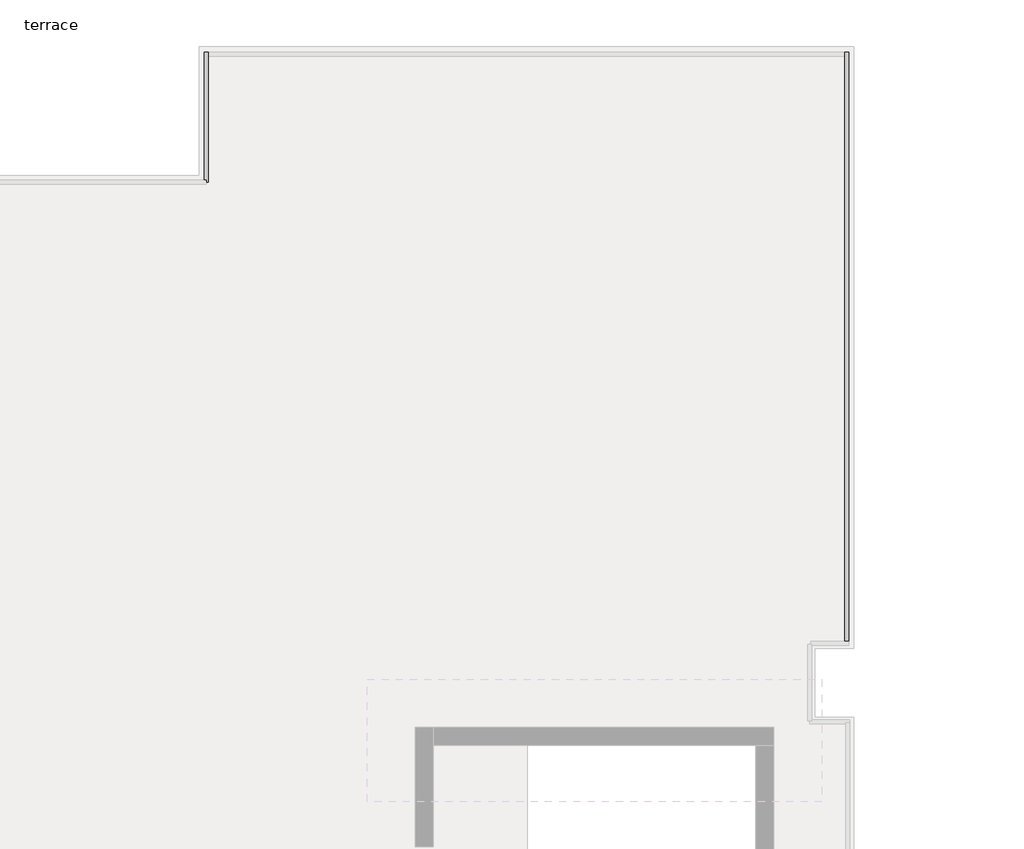
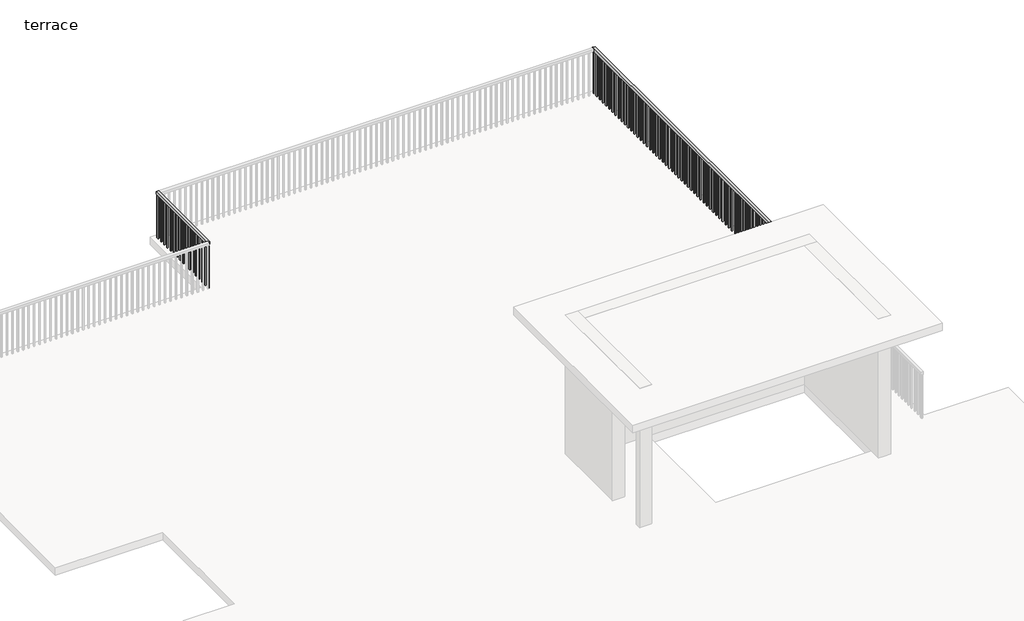
# One storey, part 6 of 7: 2 railings.
"""IFC4 building model written with IfcOpenShell, lengths in millimetres."""

from ifc_helpers import new_model, si_unit, frame, origin, place, context, project, spatial, polyline, outline, extrude, element, save

model = new_model("IFC4")

# Units and contexts
model_context = context("Model", 3, world=origin())
ifc_project = project(units=[si_unit("LENGTHUNIT", "METRE", prefix="MILLI")], contexts=[model_context])

# Site, building, storey
site = spatial("IfcSite", under=ifc_project)
building = spatial("IfcBuilding", under=site)
storey = spatial("IfcBuildingStorey", under=building, Name="terrace", Elevation=3810.0)

# Railings
placement = place(None, origin())
element("IfcRailing", 1, ObjectType="Handrail - Rectangular", at=placement, inside=storey, context=model_context, shape_type="SweptSolid", body=[
    extrude(outline(polyline([(-8384.4890129, 11008.027622), (-8435.2890129, 11008.027622), (-8435.2890129, 12659.027622), (-8384.4890129, 12659.027622), (-8384.4890129, 11008.027622)])), frame((0.0, 0.0, 4673.6), z_axis=(0.0, 0.0, 1.0), x_axis=(1.0, 0.0, 0.0)), (0.0, 0.0, 1.0), 50.8),
    extrude(outline(polyline([(-8400.3640129, 12624.102622), (-8419.4140129, 12624.102622), (-8419.4140129, 12643.152622), (-8400.3640129, 12643.152622), (-8400.3640129, 12624.102622)])), frame((0.0, 0.0, 3810.0), z_axis=(0.0, 0.0, 1.0), x_axis=(1.0, 0.0, 0.0)), (0.0, 0.0, 1.0), 863.6),
    extrude(outline(polyline([(-8400.3640129, 12522.502622), (-8419.4140129, 12522.502622), (-8419.4140129, 12541.552622), (-8400.3640129, 12541.552622), (-8400.3640129, 12522.502622)])), frame((0.0, 0.0, 3810.0), z_axis=(0.0, 0.0, 1.0), x_axis=(1.0, 0.0, 0.0)), (0.0, 0.0, 1.0), 863.6),
    extrude(outline(polyline([(-8400.3640129, 12420.902622), (-8419.4140129, 12420.902622), (-8419.4140129, 12439.952622), (-8400.3640129, 12439.952622), (-8400.3640129, 12420.902622)])), frame((0.0, 0.0, 3810.0), z_axis=(0.0, 0.0, 1.0), x_axis=(1.0, 0.0, 0.0)), (0.0, 0.0, 1.0), 863.6),
    extrude(outline(polyline([(-8400.3640129, 12319.302622), (-8419.4140129, 12319.302622), (-8419.4140129, 12338.352622), (-8400.3640129, 12338.352622), (-8400.3640129, 12319.302622)])), frame((0.0, 0.0, 3810.0), z_axis=(0.0, 0.0, 1.0), x_axis=(1.0, 0.0, 0.0)), (0.0, 0.0, 1.0), 863.6),
    extrude(outline(polyline([(-8400.3640129, 12217.702622), (-8419.4140129, 12217.702622), (-8419.4140129, 12236.752622), (-8400.3640129, 12236.752622), (-8400.3640129, 12217.702622)])), frame((0.0, 0.0, 3810.0), z_axis=(0.0, 0.0, 1.0), x_axis=(1.0, 0.0, 0.0)), (0.0, 0.0, 1.0), 863.6),
    extrude(outline(polyline([(-8400.3640129, 12116.102622), (-8419.4140129, 12116.102622), (-8419.4140129, 12135.152622), (-8400.3640129, 12135.152622), (-8400.3640129, 12116.102622)])), frame((0.0, 0.0, 3810.0), z_axis=(0.0, 0.0, 1.0), x_axis=(1.0, 0.0, 0.0)), (0.0, 0.0, 1.0), 863.6),
    extrude(outline(polyline([(-8400.3640129, 12014.502622), (-8419.4140129, 12014.502622), (-8419.4140129, 12033.552622), (-8400.3640129, 12033.552622), (-8400.3640129, 12014.502622)])), frame((0.0, 0.0, 3810.0), z_axis=(0.0, 0.0, 1.0), x_axis=(1.0, 0.0, 0.0)), (0.0, 0.0, 1.0), 863.6),
    extrude(outline(polyline([(-8400.3640129, 11912.902622), (-8419.4140129, 11912.902622), (-8419.4140129, 11931.952622), (-8400.3640129, 11931.952622), (-8400.3640129, 11912.902622)])), frame((0.0, 0.0, 3810.0), z_axis=(0.0, 0.0, 1.0), x_axis=(1.0, 0.0, 0.0)), (0.0, 0.0, 1.0), 863.6),
    extrude(outline(polyline([(-8400.3640129, 11811.302622), (-8419.4140129, 11811.302622), (-8419.4140129, 11830.352622), (-8400.3640129, 11830.352622), (-8400.3640129, 11811.302622)])), frame((0.0, 0.0, 3810.0), z_axis=(0.0, 0.0, 1.0), x_axis=(1.0, 0.0, 0.0)), (0.0, 0.0, 1.0), 863.6),
    extrude(outline(polyline([(-8400.3640129, 11709.702622), (-8419.4140129, 11709.702622), (-8419.4140129, 11728.752622), (-8400.3640129, 11728.752622), (-8400.3640129, 11709.702622)])), frame((0.0, 0.0, 3810.0), z_axis=(0.0, 0.0, 1.0), x_axis=(1.0, 0.0, 0.0)), (0.0, 0.0, 1.0), 863.6),
    extrude(outline(polyline([(-8400.3640129, 11608.102622), (-8419.4140129, 11608.102622), (-8419.4140129, 11627.152622), (-8400.3640129, 11627.152622), (-8400.3640129, 11608.102622)])), frame((0.0, 0.0, 3810.0), z_axis=(0.0, 0.0, 1.0), x_axis=(1.0, 0.0, 0.0)), (0.0, 0.0, 1.0), 863.6),
    extrude(outline(polyline([(-8400.3640129, 11506.502622), (-8419.4140129, 11506.502622), (-8419.4140129, 11525.552622), (-8400.3640129, 11525.552622), (-8400.3640129, 11506.502622)])), frame((0.0, 0.0, 3810.0), z_axis=(0.0, 0.0, 1.0), x_axis=(1.0, 0.0, 0.0)), (0.0, 0.0, 1.0), 863.6),
    extrude(outline(polyline([(-8400.3640129, 11404.902622), (-8419.4140129, 11404.902622), (-8419.4140129, 11423.952622), (-8400.3640129, 11423.952622), (-8400.3640129, 11404.902622)])), frame((0.0, 0.0, 3810.0), z_axis=(0.0, 0.0, 1.0), x_axis=(1.0, 0.0, 0.0)), (0.0, 0.0, 1.0), 863.6),
    extrude(outline(polyline([(-8400.3640129, 11303.302622), (-8419.4140129, 11303.302622), (-8419.4140129, 11322.352622), (-8400.3640129, 11322.352622), (-8400.3640129, 11303.302622)])), frame((0.0, 0.0, 3810.0), z_axis=(0.0, 0.0, 1.0), x_axis=(1.0, 0.0, 0.0)), (0.0, 0.0, 1.0), 863.6),
    extrude(outline(polyline([(-8400.3640129, 11201.702622), (-8419.4140129, 11201.702622), (-8419.4140129, 11220.752622), (-8400.3640129, 11220.752622), (-8400.3640129, 11201.702622)])), frame((0.0, 0.0, 3810.0), z_axis=(0.0, 0.0, 1.0), x_axis=(1.0, 0.0, 0.0)), (0.0, 0.0, 1.0), 863.6),
    extrude(outline(polyline([(-8400.3640129, 11100.102622), (-8419.4140129, 11100.102622), (-8419.4140129, 11119.152622), (-8400.3640129, 11119.152622), (-8400.3640129, 11100.102622)])), frame((0.0, 0.0, 3810.0), z_axis=(0.0, 0.0, 1.0), x_axis=(1.0, 0.0, 0.0)), (0.0, 0.0, 1.0), 863.6),
    extrude(outline(polyline([(-8400.3640129, 12639.977622), (-8419.4140129, 12639.977622), (-8419.4140129, 12659.027622), (-8400.3640129, 12659.027622), (-8400.3640129, 12639.977622)])), frame((0.0, 0.0, 3810.0), z_axis=(0.0, 0.0, 1.0), x_axis=(1.0, 0.0, 0.0)), (0.0, 0.0, 1.0), 863.6),
    extrude(outline(polyline([(-8400.3640129, 11008.027622), (-8419.4140129, 11008.027622), (-8419.4140129, 11027.077622), (-8400.3640129, 11027.077622), (-8400.3640129, 11008.027622)])), frame((0.0, 0.0, 3810.0), z_axis=(0.0, 0.0, 1.0), x_axis=(1.0, 0.0, 0.0)), (0.0, 0.0, 1.0), 863.6),
])
element("IfcRailing", 2, ObjectType="Handrail - Rectangular", at=placement, inside=storey, context=model_context, shape_type="SweptSolid", body=[
    extrude(outline(polyline([(-307.2890129, 12659.027622), (-256.4890129, 12659.027622), (-256.4890129, 5140.627622), (-307.2890129, 5140.627622), (-307.2890129, 12659.027622)])), frame((0.0, 0.0, 4673.6), z_axis=(0.0, 0.0, 1.0), x_axis=(1.0, 0.0, 0.0)), (0.0, 0.0, 1.0), 50.8),
    extrude(outline(polyline([(-291.4140129, 5251.752622), (-272.3640129, 5251.752622), (-272.3640129, 5232.702622), (-291.4140129, 5232.702622), (-291.4140129, 5251.752622)])), frame((0.0, 0.0, 3810.0), z_axis=(0.0, 0.0, 1.0), x_axis=(1.0, 0.0, 0.0)), (0.0, 0.0, 1.0), 863.6),
    extrude(outline(polyline([(-291.4140129, 5353.352622), (-272.3640129, 5353.352622), (-272.3640129, 5334.302622), (-291.4140129, 5334.302622), (-291.4140129, 5353.352622)])), frame((0.0, 0.0, 3810.0), z_axis=(0.0, 0.0, 1.0), x_axis=(1.0, 0.0, 0.0)), (0.0, 0.0, 1.0), 863.6),
    extrude(outline(polyline([(-291.4140129, 5454.952622), (-272.3640129, 5454.952622), (-272.3640129, 5435.902622), (-291.4140129, 5435.902622), (-291.4140129, 5454.952622)])), frame((0.0, 0.0, 3810.0), z_axis=(0.0, 0.0, 1.0), x_axis=(1.0, 0.0, 0.0)), (0.0, 0.0, 1.0), 863.6),
    extrude(outline(polyline([(-291.4140129, 5556.552622), (-272.3640129, 5556.552622), (-272.3640129, 5537.502622), (-291.4140129, 5537.502622), (-291.4140129, 5556.552622)])), frame((0.0, 0.0, 3810.0), z_axis=(0.0, 0.0, 1.0), x_axis=(1.0, 0.0, 0.0)), (0.0, 0.0, 1.0), 863.6),
    extrude(outline(polyline([(-291.4140129, 5658.152622), (-272.3640129, 5658.152622), (-272.3640129, 5639.102622), (-291.4140129, 5639.102622), (-291.4140129, 5658.152622)])), frame((0.0, 0.0, 3810.0), z_axis=(0.0, 0.0, 1.0), x_axis=(1.0, 0.0, 0.0)), (0.0, 0.0, 1.0), 863.6),
    extrude(outline(polyline([(-291.4140129, 5759.752622), (-272.3640129, 5759.752622), (-272.3640129, 5740.702622), (-291.4140129, 5740.702622), (-291.4140129, 5759.752622)])), frame((0.0, 0.0, 3810.0), z_axis=(0.0, 0.0, 1.0), x_axis=(1.0, 0.0, 0.0)), (0.0, 0.0, 1.0), 863.6),
    extrude(outline(polyline([(-291.4140129, 5861.352622), (-272.3640129, 5861.352622), (-272.3640129, 5842.302622), (-291.4140129, 5842.302622), (-291.4140129, 5861.352622)])), frame((0.0, 0.0, 3810.0), z_axis=(0.0, 0.0, 1.0), x_axis=(1.0, 0.0, 0.0)), (0.0, 0.0, 1.0), 863.6),
    extrude(outline(polyline([(-291.4140129, 5962.952622), (-272.3640129, 5962.952622), (-272.3640129, 5943.902622), (-291.4140129, 5943.902622), (-291.4140129, 5962.952622)])), frame((0.0, 0.0, 3810.0), z_axis=(0.0, 0.0, 1.0), x_axis=(1.0, 0.0, 0.0)), (0.0, 0.0, 1.0), 863.6),
    extrude(outline(polyline([(-291.4140129, 6064.552622), (-272.3640129, 6064.552622), (-272.3640129, 6045.502622), (-291.4140129, 6045.502622), (-291.4140129, 6064.552622)])), frame((0.0, 0.0, 3810.0), z_axis=(0.0, 0.0, 1.0), x_axis=(1.0, 0.0, 0.0)), (0.0, 0.0, 1.0), 863.6),
    extrude(outline(polyline([(-291.4140129, 6166.152622), (-272.3640129, 6166.152622), (-272.3640129, 6147.102622), (-291.4140129, 6147.102622), (-291.4140129, 6166.152622)])), frame((0.0, 0.0, 3810.0), z_axis=(0.0, 0.0, 1.0), x_axis=(1.0, 0.0, 0.0)), (0.0, 0.0, 1.0), 863.6),
    extrude(outline(polyline([(-291.4140129, 6267.752622), (-272.3640129, 6267.752622), (-272.3640129, 6248.702622), (-291.4140129, 6248.702622), (-291.4140129, 6267.752622)])), frame((0.0, 0.0, 3810.0), z_axis=(0.0, 0.0, 1.0), x_axis=(1.0, 0.0, 0.0)), (0.0, 0.0, 1.0), 863.6),
    extrude(outline(polyline([(-291.4140129, 6369.352622), (-272.3640129, 6369.352622), (-272.3640129, 6350.302622), (-291.4140129, 6350.302622), (-291.4140129, 6369.352622)])), frame((0.0, 0.0, 3810.0), z_axis=(0.0, 0.0, 1.0), x_axis=(1.0, 0.0, 0.0)), (0.0, 0.0, 1.0), 863.6),
    extrude(outline(polyline([(-291.4140129, 6470.952622), (-272.3640129, 6470.952622), (-272.3640129, 6451.902622), (-291.4140129, 6451.902622), (-291.4140129, 6470.952622)])), frame((0.0, 0.0, 3810.0), z_axis=(0.0, 0.0, 1.0), x_axis=(1.0, 0.0, 0.0)), (0.0, 0.0, 1.0), 863.6),
    extrude(outline(polyline([(-291.4140129, 6572.552622), (-272.3640129, 6572.552622), (-272.3640129, 6553.502622), (-291.4140129, 6553.502622), (-291.4140129, 6572.552622)])), frame((0.0, 0.0, 3810.0), z_axis=(0.0, 0.0, 1.0), x_axis=(1.0, 0.0, 0.0)), (0.0, 0.0, 1.0), 863.6),
    extrude(outline(polyline([(-291.4140129, 6674.152622), (-272.3640129, 6674.152622), (-272.3640129, 6655.102622), (-291.4140129, 6655.102622), (-291.4140129, 6674.152622)])), frame((0.0, 0.0, 3810.0), z_axis=(0.0, 0.0, 1.0), x_axis=(1.0, 0.0, 0.0)), (0.0, 0.0, 1.0), 863.6),
    extrude(outline(polyline([(-291.4140129, 6775.752622), (-272.3640129, 6775.752622), (-272.3640129, 6756.702622), (-291.4140129, 6756.702622), (-291.4140129, 6775.752622)])), frame((0.0, 0.0, 3810.0), z_axis=(0.0, 0.0, 1.0), x_axis=(1.0, 0.0, 0.0)), (0.0, 0.0, 1.0), 863.6),
    extrude(outline(polyline([(-291.4140129, 6877.352622), (-272.3640129, 6877.352622), (-272.3640129, 6858.302622), (-291.4140129, 6858.302622), (-291.4140129, 6877.352622)])), frame((0.0, 0.0, 3810.0), z_axis=(0.0, 0.0, 1.0), x_axis=(1.0, 0.0, 0.0)), (0.0, 0.0, 1.0), 863.6),
    extrude(outline(polyline([(-291.4140129, 6978.952622), (-272.3640129, 6978.952622), (-272.3640129, 6959.902622), (-291.4140129, 6959.902622), (-291.4140129, 6978.952622)])), frame((0.0, 0.0, 3810.0), z_axis=(0.0, 0.0, 1.0), x_axis=(1.0, 0.0, 0.0)), (0.0, 0.0, 1.0), 863.6),
    extrude(outline(polyline([(-291.4140129, 7080.552622), (-272.3640129, 7080.552622), (-272.3640129, 7061.502622), (-291.4140129, 7061.502622), (-291.4140129, 7080.552622)])), frame((0.0, 0.0, 3810.0), z_axis=(0.0, 0.0, 1.0), x_axis=(1.0, 0.0, 0.0)), (0.0, 0.0, 1.0), 863.6),
    extrude(outline(polyline([(-291.4140129, 7182.152622), (-272.3640129, 7182.152622), (-272.3640129, 7163.102622), (-291.4140129, 7163.102622), (-291.4140129, 7182.152622)])), frame((0.0, 0.0, 3810.0), z_axis=(0.0, 0.0, 1.0), x_axis=(1.0, 0.0, 0.0)), (0.0, 0.0, 1.0), 863.6),
    extrude(outline(polyline([(-291.4140129, 7283.752622), (-272.3640129, 7283.752622), (-272.3640129, 7264.702622), (-291.4140129, 7264.702622), (-291.4140129, 7283.752622)])), frame((0.0, 0.0, 3810.0), z_axis=(0.0, 0.0, 1.0), x_axis=(1.0, 0.0, 0.0)), (0.0, 0.0, 1.0), 863.6),
    extrude(outline(polyline([(-291.4140129, 7385.352622), (-272.3640129, 7385.352622), (-272.3640129, 7366.302622), (-291.4140129, 7366.302622), (-291.4140129, 7385.352622)])), frame((0.0, 0.0, 3810.0), z_axis=(0.0, 0.0, 1.0), x_axis=(1.0, 0.0, 0.0)), (0.0, 0.0, 1.0), 863.6),
    extrude(outline(polyline([(-291.4140129, 7486.952622), (-272.3640129, 7486.952622), (-272.3640129, 7467.902622), (-291.4140129, 7467.902622), (-291.4140129, 7486.952622)])), frame((0.0, 0.0, 3810.0), z_axis=(0.0, 0.0, 1.0), x_axis=(1.0, 0.0, 0.0)), (0.0, 0.0, 1.0), 863.6),
    extrude(outline(polyline([(-291.4140129, 7588.552622), (-272.3640129, 7588.552622), (-272.3640129, 7569.502622), (-291.4140129, 7569.502622), (-291.4140129, 7588.552622)])), frame((0.0, 0.0, 3810.0), z_axis=(0.0, 0.0, 1.0), x_axis=(1.0, 0.0, 0.0)), (0.0, 0.0, 1.0), 863.6),
    extrude(outline(polyline([(-291.4140129, 7690.152622), (-272.3640129, 7690.152622), (-272.3640129, 7671.102622), (-291.4140129, 7671.102622), (-291.4140129, 7690.152622)])), frame((0.0, 0.0, 3810.0), z_axis=(0.0, 0.0, 1.0), x_axis=(1.0, 0.0, 0.0)), (0.0, 0.0, 1.0), 863.6),
    extrude(outline(polyline([(-291.4140129, 7791.752622), (-272.3640129, 7791.752622), (-272.3640129, 7772.702622), (-291.4140129, 7772.702622), (-291.4140129, 7791.752622)])), frame((0.0, 0.0, 3810.0), z_axis=(0.0, 0.0, 1.0), x_axis=(1.0, 0.0, 0.0)), (0.0, 0.0, 1.0), 863.6),
    extrude(outline(polyline([(-291.4140129, 7893.352622), (-272.3640129, 7893.352622), (-272.3640129, 7874.302622), (-291.4140129, 7874.302622), (-291.4140129, 7893.352622)])), frame((0.0, 0.0, 3810.0), z_axis=(0.0, 0.0, 1.0), x_axis=(1.0, 0.0, 0.0)), (0.0, 0.0, 1.0), 863.6),
    extrude(outline(polyline([(-291.4140129, 7994.952622), (-272.3640129, 7994.952622), (-272.3640129, 7975.902622), (-291.4140129, 7975.902622), (-291.4140129, 7994.952622)])), frame((0.0, 0.0, 3810.0), z_axis=(0.0, 0.0, 1.0), x_axis=(1.0, 0.0, 0.0)), (0.0, 0.0, 1.0), 863.6),
    extrude(outline(polyline([(-291.4140129, 8096.552622), (-272.3640129, 8096.552622), (-272.3640129, 8077.502622), (-291.4140129, 8077.502622), (-291.4140129, 8096.552622)])), frame((0.0, 0.0, 3810.0), z_axis=(0.0, 0.0, 1.0), x_axis=(1.0, 0.0, 0.0)), (0.0, 0.0, 1.0), 863.6),
    extrude(outline(polyline([(-291.4140129, 8198.152622), (-272.3640129, 8198.152622), (-272.3640129, 8179.102622), (-291.4140129, 8179.102622), (-291.4140129, 8198.152622)])), frame((0.0, 0.0, 3810.0), z_axis=(0.0, 0.0, 1.0), x_axis=(1.0, 0.0, 0.0)), (0.0, 0.0, 1.0), 863.6),
    extrude(outline(polyline([(-291.4140129, 8299.752622), (-272.3640129, 8299.752622), (-272.3640129, 8280.702622), (-291.4140129, 8280.702622), (-291.4140129, 8299.752622)])), frame((0.0, 0.0, 3810.0), z_axis=(0.0, 0.0, 1.0), x_axis=(1.0, 0.0, 0.0)), (0.0, 0.0, 1.0), 863.6),
    extrude(outline(polyline([(-291.4140129, 8401.352622), (-272.3640129, 8401.352622), (-272.3640129, 8382.302622), (-291.4140129, 8382.302622), (-291.4140129, 8401.352622)])), frame((0.0, 0.0, 3810.0), z_axis=(0.0, 0.0, 1.0), x_axis=(1.0, 0.0, 0.0)), (0.0, 0.0, 1.0), 863.6),
    extrude(outline(polyline([(-291.4140129, 8502.952622), (-272.3640129, 8502.952622), (-272.3640129, 8483.902622), (-291.4140129, 8483.902622), (-291.4140129, 8502.952622)])), frame((0.0, 0.0, 3810.0), z_axis=(0.0, 0.0, 1.0), x_axis=(1.0, 0.0, 0.0)), (0.0, 0.0, 1.0), 863.6),
    extrude(outline(polyline([(-291.4140129, 8604.552622), (-272.3640129, 8604.552622), (-272.3640129, 8585.502622), (-291.4140129, 8585.502622), (-291.4140129, 8604.552622)])), frame((0.0, 0.0, 3810.0), z_axis=(0.0, 0.0, 1.0), x_axis=(1.0, 0.0, 0.0)), (0.0, 0.0, 1.0), 863.6),
    extrude(outline(polyline([(-291.4140129, 8706.152622), (-272.3640129, 8706.152622), (-272.3640129, 8687.102622), (-291.4140129, 8687.102622), (-291.4140129, 8706.152622)])), frame((0.0, 0.0, 3810.0), z_axis=(0.0, 0.0, 1.0), x_axis=(1.0, 0.0, 0.0)), (0.0, 0.0, 1.0), 863.6),
    extrude(outline(polyline([(-291.4140129, 8807.752622), (-272.3640129, 8807.752622), (-272.3640129, 8788.702622), (-291.4140129, 8788.702622), (-291.4140129, 8807.752622)])), frame((0.0, 0.0, 3810.0), z_axis=(0.0, 0.0, 1.0), x_axis=(1.0, 0.0, 0.0)), (0.0, 0.0, 1.0), 863.6),
    extrude(outline(polyline([(-291.4140129, 8909.352622), (-272.3640129, 8909.352622), (-272.3640129, 8890.302622), (-291.4140129, 8890.302622), (-291.4140129, 8909.352622)])), frame((0.0, 0.0, 3810.0), z_axis=(0.0, 0.0, 1.0), x_axis=(1.0, 0.0, 0.0)), (0.0, 0.0, 1.0), 863.6),
    extrude(outline(polyline([(-291.4140129, 9010.952622), (-272.3640129, 9010.952622), (-272.3640129, 8991.902622), (-291.4140129, 8991.902622), (-291.4140129, 9010.952622)])), frame((0.0, 0.0, 3810.0), z_axis=(0.0, 0.0, 1.0), x_axis=(1.0, 0.0, 0.0)), (0.0, 0.0, 1.0), 863.6),
    extrude(outline(polyline([(-291.4140129, 9112.552622), (-272.3640129, 9112.552622), (-272.3640129, 9093.502622), (-291.4140129, 9093.502622), (-291.4140129, 9112.552622)])), frame((0.0, 0.0, 3810.0), z_axis=(0.0, 0.0, 1.0), x_axis=(1.0, 0.0, 0.0)), (0.0, 0.0, 1.0), 863.6),
    extrude(outline(polyline([(-291.4140129, 9214.152622), (-272.3640129, 9214.152622), (-272.3640129, 9195.102622), (-291.4140129, 9195.102622), (-291.4140129, 9214.152622)])), frame((0.0, 0.0, 3810.0), z_axis=(0.0, 0.0, 1.0), x_axis=(1.0, 0.0, 0.0)), (0.0, 0.0, 1.0), 863.6),
    extrude(outline(polyline([(-291.4140129, 9315.752622), (-272.3640129, 9315.752622), (-272.3640129, 9296.702622), (-291.4140129, 9296.702622), (-291.4140129, 9315.752622)])), frame((0.0, 0.0, 3810.0), z_axis=(0.0, 0.0, 1.0), x_axis=(1.0, 0.0, 0.0)), (0.0, 0.0, 1.0), 863.6),
    extrude(outline(polyline([(-291.4140129, 9417.352622), (-272.3640129, 9417.352622), (-272.3640129, 9398.302622), (-291.4140129, 9398.302622), (-291.4140129, 9417.352622)])), frame((0.0, 0.0, 3810.0), z_axis=(0.0, 0.0, 1.0), x_axis=(1.0, 0.0, 0.0)), (0.0, 0.0, 1.0), 863.6),
    extrude(outline(polyline([(-291.4140129, 9518.952622), (-272.3640129, 9518.952622), (-272.3640129, 9499.902622), (-291.4140129, 9499.902622), (-291.4140129, 9518.952622)])), frame((0.0, 0.0, 3810.0), z_axis=(0.0, 0.0, 1.0), x_axis=(1.0, 0.0, 0.0)), (0.0, 0.0, 1.0), 863.6),
    extrude(outline(polyline([(-291.4140129, 9620.552622), (-272.3640129, 9620.552622), (-272.3640129, 9601.502622), (-291.4140129, 9601.502622), (-291.4140129, 9620.552622)])), frame((0.0, 0.0, 3810.0), z_axis=(0.0, 0.0, 1.0), x_axis=(1.0, 0.0, 0.0)), (0.0, 0.0, 1.0), 863.6),
    extrude(outline(polyline([(-291.4140129, 9722.152622), (-272.3640129, 9722.152622), (-272.3640129, 9703.102622), (-291.4140129, 9703.102622), (-291.4140129, 9722.152622)])), frame((0.0, 0.0, 3810.0), z_axis=(0.0, 0.0, 1.0), x_axis=(1.0, 0.0, 0.0)), (0.0, 0.0, 1.0), 863.6),
    extrude(outline(polyline([(-291.4140129, 9823.752622), (-272.3640129, 9823.752622), (-272.3640129, 9804.702622), (-291.4140129, 9804.702622), (-291.4140129, 9823.752622)])), frame((0.0, 0.0, 3810.0), z_axis=(0.0, 0.0, 1.0), x_axis=(1.0, 0.0, 0.0)), (0.0, 0.0, 1.0), 863.6),
    extrude(outline(polyline([(-291.4140129, 9925.352622), (-272.3640129, 9925.352622), (-272.3640129, 9906.302622), (-291.4140129, 9906.302622), (-291.4140129, 9925.352622)])), frame((0.0, 0.0, 3810.0), z_axis=(0.0, 0.0, 1.0), x_axis=(1.0, 0.0, 0.0)), (0.0, 0.0, 1.0), 863.6),
    extrude(outline(polyline([(-291.4140129, 10026.952622), (-272.3640129, 10026.952622), (-272.3640129, 10007.902622), (-291.4140129, 10007.902622), (-291.4140129, 10026.952622)])), frame((0.0, 0.0, 3810.0), z_axis=(0.0, 0.0, 1.0), x_axis=(1.0, 0.0, 0.0)), (0.0, 0.0, 1.0), 863.6),
    extrude(outline(polyline([(-291.4140129, 10128.552622), (-272.3640129, 10128.552622), (-272.3640129, 10109.502622), (-291.4140129, 10109.502622), (-291.4140129, 10128.552622)])), frame((0.0, 0.0, 3810.0), z_axis=(0.0, 0.0, 1.0), x_axis=(1.0, 0.0, 0.0)), (0.0, 0.0, 1.0), 863.6),
    extrude(outline(polyline([(-291.4140129, 10230.152622), (-272.3640129, 10230.152622), (-272.3640129, 10211.102622), (-291.4140129, 10211.102622), (-291.4140129, 10230.152622)])), frame((0.0, 0.0, 3810.0), z_axis=(0.0, 0.0, 1.0), x_axis=(1.0, 0.0, 0.0)), (0.0, 0.0, 1.0), 863.6),
    extrude(outline(polyline([(-291.4140129, 10331.752622), (-272.3640129, 10331.752622), (-272.3640129, 10312.702622), (-291.4140129, 10312.702622), (-291.4140129, 10331.752622)])), frame((0.0, 0.0, 3810.0), z_axis=(0.0, 0.0, 1.0), x_axis=(1.0, 0.0, 0.0)), (0.0, 0.0, 1.0), 863.6),
    extrude(outline(polyline([(-291.4140129, 10433.352622), (-272.3640129, 10433.352622), (-272.3640129, 10414.302622), (-291.4140129, 10414.302622), (-291.4140129, 10433.352622)])), frame((0.0, 0.0, 3810.0), z_axis=(0.0, 0.0, 1.0), x_axis=(1.0, 0.0, 0.0)), (0.0, 0.0, 1.0), 863.6),
    extrude(outline(polyline([(-291.4140129, 10534.952622), (-272.3640129, 10534.952622), (-272.3640129, 10515.902622), (-291.4140129, 10515.902622), (-291.4140129, 10534.952622)])), frame((0.0, 0.0, 3810.0), z_axis=(0.0, 0.0, 1.0), x_axis=(1.0, 0.0, 0.0)), (0.0, 0.0, 1.0), 863.6),
    extrude(outline(polyline([(-291.4140129, 10636.552622), (-272.3640129, 10636.552622), (-272.3640129, 10617.502622), (-291.4140129, 10617.502622), (-291.4140129, 10636.552622)])), frame((0.0, 0.0, 3810.0), z_axis=(0.0, 0.0, 1.0), x_axis=(1.0, 0.0, 0.0)), (0.0, 0.0, 1.0), 863.6),
    extrude(outline(polyline([(-291.4140129, 10738.152622), (-272.3640129, 10738.152622), (-272.3640129, 10719.102622), (-291.4140129, 10719.102622), (-291.4140129, 10738.152622)])), frame((0.0, 0.0, 3810.0), z_axis=(0.0, 0.0, 1.0), x_axis=(1.0, 0.0, 0.0)), (0.0, 0.0, 1.0), 863.6),
    extrude(outline(polyline([(-291.4140129, 10839.752622), (-272.3640129, 10839.752622), (-272.3640129, 10820.702622), (-291.4140129, 10820.702622), (-291.4140129, 10839.752622)])), frame((0.0, 0.0, 3810.0), z_axis=(0.0, 0.0, 1.0), x_axis=(1.0, 0.0, 0.0)), (0.0, 0.0, 1.0), 863.6),
    extrude(outline(polyline([(-291.4140129, 10941.352622), (-272.3640129, 10941.352622), (-272.3640129, 10922.302622), (-291.4140129, 10922.302622), (-291.4140129, 10941.352622)])), frame((0.0, 0.0, 3810.0), z_axis=(0.0, 0.0, 1.0), x_axis=(1.0, 0.0, 0.0)), (0.0, 0.0, 1.0), 863.6),
    extrude(outline(polyline([(-291.4140129, 11042.952622), (-272.3640129, 11042.952622), (-272.3640129, 11023.902622), (-291.4140129, 11023.902622), (-291.4140129, 11042.952622)])), frame((0.0, 0.0, 3810.0), z_axis=(0.0, 0.0, 1.0), x_axis=(1.0, 0.0, 0.0)), (0.0, 0.0, 1.0), 863.6),
    extrude(outline(polyline([(-291.4140129, 11144.552622), (-272.3640129, 11144.552622), (-272.3640129, 11125.502622), (-291.4140129, 11125.502622), (-291.4140129, 11144.552622)])), frame((0.0, 0.0, 3810.0), z_axis=(0.0, 0.0, 1.0), x_axis=(1.0, 0.0, 0.0)), (0.0, 0.0, 1.0), 863.6),
    extrude(outline(polyline([(-291.4140129, 11246.152622), (-272.3640129, 11246.152622), (-272.3640129, 11227.102622), (-291.4140129, 11227.102622), (-291.4140129, 11246.152622)])), frame((0.0, 0.0, 3810.0), z_axis=(0.0, 0.0, 1.0), x_axis=(1.0, 0.0, 0.0)), (0.0, 0.0, 1.0), 863.6),
    extrude(outline(polyline([(-291.4140129, 11347.752622), (-272.3640129, 11347.752622), (-272.3640129, 11328.702622), (-291.4140129, 11328.702622), (-291.4140129, 11347.752622)])), frame((0.0, 0.0, 3810.0), z_axis=(0.0, 0.0, 1.0), x_axis=(1.0, 0.0, 0.0)), (0.0, 0.0, 1.0), 863.6),
    extrude(outline(polyline([(-291.4140129, 11449.352622), (-272.3640129, 11449.352622), (-272.3640129, 11430.302622), (-291.4140129, 11430.302622), (-291.4140129, 11449.352622)])), frame((0.0, 0.0, 3810.0), z_axis=(0.0, 0.0, 1.0), x_axis=(1.0, 0.0, 0.0)), (0.0, 0.0, 1.0), 863.6),
    extrude(outline(polyline([(-291.4140129, 11550.952622), (-272.3640129, 11550.952622), (-272.3640129, 11531.902622), (-291.4140129, 11531.902622), (-291.4140129, 11550.952622)])), frame((0.0, 0.0, 3810.0), z_axis=(0.0, 0.0, 1.0), x_axis=(1.0, 0.0, 0.0)), (0.0, 0.0, 1.0), 863.6),
    extrude(outline(polyline([(-291.4140129, 11652.552622), (-272.3640129, 11652.552622), (-272.3640129, 11633.502622), (-291.4140129, 11633.502622), (-291.4140129, 11652.552622)])), frame((0.0, 0.0, 3810.0), z_axis=(0.0, 0.0, 1.0), x_axis=(1.0, 0.0, 0.0)), (0.0, 0.0, 1.0), 863.6),
    extrude(outline(polyline([(-291.4140129, 11754.152622), (-272.3640129, 11754.152622), (-272.3640129, 11735.102622), (-291.4140129, 11735.102622), (-291.4140129, 11754.152622)])), frame((0.0, 0.0, 3810.0), z_axis=(0.0, 0.0, 1.0), x_axis=(1.0, 0.0, 0.0)), (0.0, 0.0, 1.0), 863.6),
    extrude(outline(polyline([(-291.4140129, 11855.752622), (-272.3640129, 11855.752622), (-272.3640129, 11836.702622), (-291.4140129, 11836.702622), (-291.4140129, 11855.752622)])), frame((0.0, 0.0, 3810.0), z_axis=(0.0, 0.0, 1.0), x_axis=(1.0, 0.0, 0.0)), (0.0, 0.0, 1.0), 863.6),
    extrude(outline(polyline([(-291.4140129, 11957.352622), (-272.3640129, 11957.352622), (-272.3640129, 11938.302622), (-291.4140129, 11938.302622), (-291.4140129, 11957.352622)])), frame((0.0, 0.0, 3810.0), z_axis=(0.0, 0.0, 1.0), x_axis=(1.0, 0.0, 0.0)), (0.0, 0.0, 1.0), 863.6),
    extrude(outline(polyline([(-291.4140129, 12058.952622), (-272.3640129, 12058.952622), (-272.3640129, 12039.902622), (-291.4140129, 12039.902622), (-291.4140129, 12058.952622)])), frame((0.0, 0.0, 3810.0), z_axis=(0.0, 0.0, 1.0), x_axis=(1.0, 0.0, 0.0)), (0.0, 0.0, 1.0), 863.6),
    extrude(outline(polyline([(-291.4140129, 12160.552622), (-272.3640129, 12160.552622), (-272.3640129, 12141.502622), (-291.4140129, 12141.502622), (-291.4140129, 12160.552622)])), frame((0.0, 0.0, 3810.0), z_axis=(0.0, 0.0, 1.0), x_axis=(1.0, 0.0, 0.0)), (0.0, 0.0, 1.0), 863.6),
    extrude(outline(polyline([(-291.4140129, 12262.152622), (-272.3640129, 12262.152622), (-272.3640129, 12243.102622), (-291.4140129, 12243.102622), (-291.4140129, 12262.152622)])), frame((0.0, 0.0, 3810.0), z_axis=(0.0, 0.0, 1.0), x_axis=(1.0, 0.0, 0.0)), (0.0, 0.0, 1.0), 863.6),
    extrude(outline(polyline([(-291.4140129, 12363.752622), (-272.3640129, 12363.752622), (-272.3640129, 12344.702622), (-291.4140129, 12344.702622), (-291.4140129, 12363.752622)])), frame((0.0, 0.0, 3810.0), z_axis=(0.0, 0.0, 1.0), x_axis=(1.0, 0.0, 0.0)), (0.0, 0.0, 1.0), 863.6),
    extrude(outline(polyline([(-291.4140129, 12465.352622), (-272.3640129, 12465.352622), (-272.3640129, 12446.302622), (-291.4140129, 12446.302622), (-291.4140129, 12465.352622)])), frame((0.0, 0.0, 3810.0), z_axis=(0.0, 0.0, 1.0), x_axis=(1.0, 0.0, 0.0)), (0.0, 0.0, 1.0), 863.6),
    extrude(outline(polyline([(-291.4140129, 12566.952622), (-272.3640129, 12566.952622), (-272.3640129, 12547.902622), (-291.4140129, 12547.902622), (-291.4140129, 12566.952622)])), frame((0.0, 0.0, 3810.0), z_axis=(0.0, 0.0, 1.0), x_axis=(1.0, 0.0, 0.0)), (0.0, 0.0, 1.0), 863.6),
    extrude(outline(polyline([(-291.4140129, 5159.677622), (-272.3640129, 5159.677622), (-272.3640129, 5140.627622), (-291.4140129, 5140.627622), (-291.4140129, 5159.677622)])), frame((0.0, 0.0, 3810.0), z_axis=(0.0, 0.0, 1.0), x_axis=(1.0, 0.0, 0.0)), (0.0, 0.0, 1.0), 863.6),
    extrude(outline(polyline([(-291.4140129, 12659.027622), (-272.3640129, 12659.027622), (-272.3640129, 12639.977622), (-291.4140129, 12639.977622), (-291.4140129, 12659.027622)])), frame((0.0, 0.0, 3810.0), z_axis=(0.0, 0.0, 1.0), x_axis=(1.0, 0.0, 0.0)), (0.0, 0.0, 1.0), 863.6),
])

save(model, "model.ifc")

# Revit data of these elements
# Type "Handrail - Rectangular"
#   Assembly Code = "C2010400"
#   built-in parameter 1008612 = 0.0416667 (stored number, unit not read)
#   built-in parameter 1008611 = 0.0416667 (stored number, unit not read)
#   built-in parameter 1008609 = 0.333333 (stored number, unit not read)
#   built-in parameter 1008604 = 0.166667 (stored number, unit not read)
#   built-in parameter 1008603 = 0.166667 (stored number, unit not read)
#   Railing Height = 3' - 0"
#   built-in parameter 1008630 = 2
#   built-in parameter 1008610 = 2
#   built-in parameter 1008618 = Baluster - Square : 3/4"
# Elements 1, 2 (IfcRailing, "Handrail - Rectangular")
#   Phase Created = New Construction
